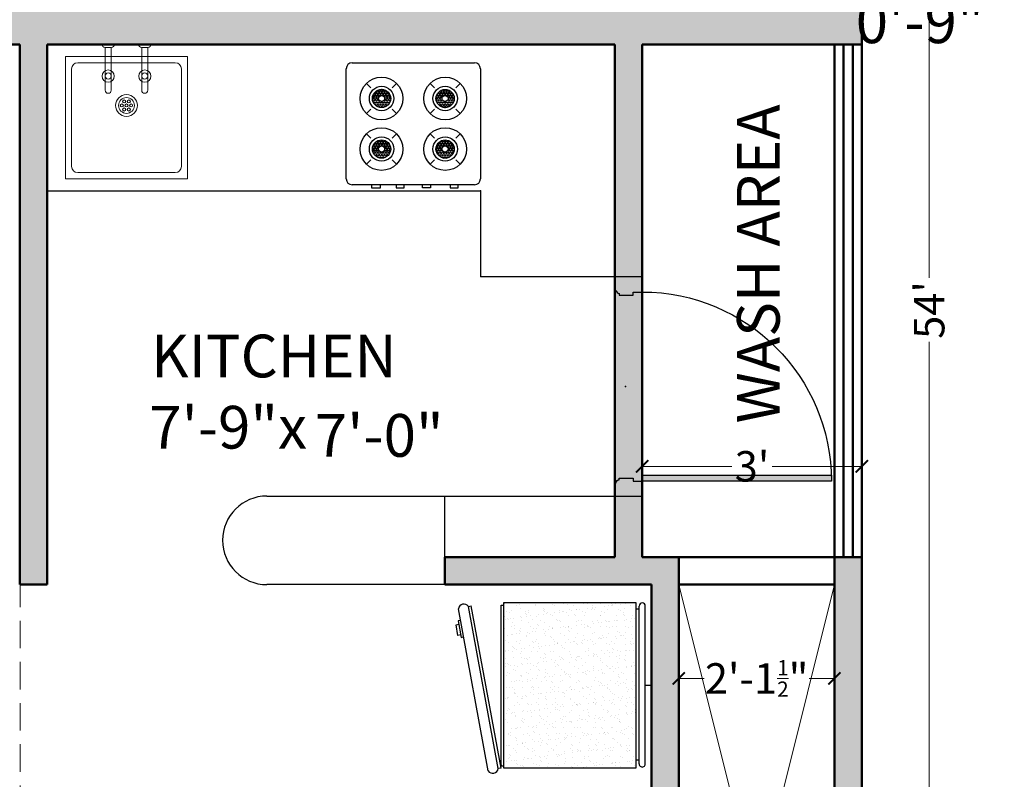
# Model space of a CAD drawing. Units: inches. Extents: x 4508 to 5907, y 877 to 1592.
# Tile 12 of 20: x 5392 to 5553, y 1174 to 1298. Entities that reach past the tile are written whole.
import ezdxf

# ---------------------------------------------------------------- set-up
doc = ezdxf.new("R2010")
doc.units = ezdxf.units.IN
doc.linetypes.add('DASHED', pattern=[0.75, 0.5, -0.25])
doc.layers.get('DEFPOINTS').update_dxf_attribs({"color": 8})
for name, color, linetype, lineweight in [('A-ANNO-DIMS', 2, 'Continuous', 18), ('A-ANNO-TEXT', 7, 'Continuous', 25), ('A-DOOR', 4, 'Continuous', 25), ('A-FLOR-CASE', 30, 'Continuous', 25), ('A-FLOR-FIXT', 8, 'Continuous', 18), ('A-FLOR-OVHD', 5, 'DASHED', 18), ('A-FLOR-SHFT', 8, 'Continuous', 18), ('A-WALL', 7, 'Continuous', 50), ('A-WALL-PATT', 8, 'Continuous', 13)]:
    doc.layers.add(name, color=color, linetype=linetype, lineweight=lineweight)
doc.layers.add('doors & windows', color=30, linetype='Continuous')
doc.layers.add('furniture', color=24, linetype='Continuous')
doc.styles.get("Standard").update_dxf_attribs({"font": 'arial.ttf'})
doc.dimstyles.new('details', dxfattribs={"dimtxt": 5, "dimasz": 2, "dimexe": 2, "dimexo": 3, "dimgap": 1, "dimtad": 0, "dimdec": 1, "dimzin": 0, "dimdsep": 46, "dimlunit": 4, "dimtxsty": 'Standard', "dimblk": 'ARCHTICK', "dimcen": 3, "dimclrd": 256, "dimclre": 256, "dimclrt": 256, "dimadec": 0, "dimazin": 0, "dimtfac": 0.5, "dimtdec": 1, "dimtofl": 0, "dimtmove": 0, "dimatfit": 3, "dimldrblk": 'CLOSEDBLANK', "dimfxl": 2, "dimtolj": 1, "dimtzin": 0, "dimlwd": -1, "dimlwe": -1, "dimarcsym": 0})
doc.dimstyles.new('text', dxfattribs={"dimtxt": 7, "dimasz": 0, "dimexe": 3, "dimexo": 3, "dimgap": 0, "dimtad": 1, "dimtih": 1, "dimtoh": 1, "dimzin": 3, "dimdsep": 46, "dimlunit": 4, "dimtxsty": 'Standard', "dimblk": 'CLOSEDBLANK', "dimcen": 3, "dimse1": 1, "dimse2": 1, "dimsd1": 1, "dimsd2": 1, "dimclrd": 256, "dimclre": 256, "dimclrt": 256, "dimadec": 0, "dimazin": 0, "dimtfac": 0.5, "dimtofl": 0, "dimtmove": 0, "dimatfit": 3, "dimfxl": 3, "dimtolj": 1, "dimtzin": 0, "dimlwd": -1, "dimlwe": -1, "dimarcsym": 0})

# ---------------------------------------------------------------- blocks, each defined once
blk = doc.blocks.new('_ArchTick')
at = {"color": 0, "linetype": 'ByBlock', "const_width": 0.15}
blk.add_lwpolyline([(-0.5, -0.5), (0.5, 0.5)], dxfattribs=at)
blk = doc.blocks.new('*D92')
at = {"layer": 'A-ANNO-DIMS', "color": 0, "transparency": 16777216}
for p, q in [((5499.9, 1202.7), (5499.9, 1188.32)), ((5525.4, 1202.7), (5525.4, 1188.32)), ((5499.9, 1190.32), (5504.05, 1190.32)), ((5525.4, 1190.32), (5521.25, 1190.32))]:
    blk.add_line(p, q, dxfattribs=at)
at = {"layer": 'DEFPOINTS', "color": 0, "transparency": 16777216}
for p in [(5499.9, 1205.7), (5525.4, 1205.7), (5499.9, 1190.32)]:
    blk.add_point(p, dxfattribs=at)
at = {"layer": 'A-ANNO-DIMS', "color": 0, "transparency": 16777216, "xscale": 2, "yscale": 2, "zscale": 2, "rotation": 180}
blk.add_blockref('_ArchTick', (5499.9, 1190.32), dxfattribs=at)
at = {"layer": 'A-ANNO-DIMS', "color": 0, "transparency": 16777216, "xscale": 2, "yscale": 2, "zscale": 2}
blk.add_blockref('_ArchTick', (5525.4, 1190.32), dxfattribs=at)
at = {"layer": 'A-ANNO-DIMS', "color": 0, "transparency": 16777216, "insert": (5512.65, 1190.32), "char_height": 5, "attachment_point": 5}
blk.add_mtext('\\A1;2\'-1{\\H0.5x;\\S1/2;}"', dxfattribs=at)
blk = doc.blocks.new('_ClosedBlank')
at = {"color": 0, "lineweight": -2}
for p, q in [((-1, 0.167), (0, 0)), ((-1, 0.167), (-1, -0.167)), ((0, 0), (-1, -0.167))]:
    blk.add_line(p, q, dxfattribs=at)
blk = doc.blocks.new('D1')
at = {"layer": 'doors & windows'}
h = blk.add_hatch(dxfattribs=at)
h.set_pattern_fill('DOTS', color=256, scale=2, angle=180, style=0)
h.set_pattern_definition([(180, (-2e-12, -4), (-0.0625, -0.125), [0, -0.125])])
h.paths.add_polyline_path([(2.5, 0), (3.5, 0), (3.5, 30.98, 0.008066), (2.5, 31)])
h = blk.add_hatch(dxfattribs=at)
h.set_pattern_fill('DOTS', color=256, scale=2, angle=180, style=0)
h.set_pattern_definition([(180, (0, -0.5), (-0.0625, -0.125), [0, -0.125])])
h.paths.add_polyline_path([(0, -4.5), (2.25, -4.5), (2.25, -4.25, 0.403966), (2.75, -3.75), (3, -3.75), (3, -1.5), (2.5, -1.5), (2.5, 0), (0, 0)])
h.paths.add_polyline_path([(36, -4.5), (36, 0), (33.5, 0), (33.5, -1.5), (33, -1.5), (33, -3.75), (33.25, -3.75, 0.403966), (33.75, -4.25), (33.75, -4.5)])
for p, q in [((0, 0), (0, -4.5)), ((36, 0), (36, -4.5))]:
    blk.add_line(p, q)
blk.add_lwpolyline([(3.5, 0), (3.5, 31), (2.5, 31), (2.5, 0)], close=True, dxfattribs=at)
for points in [[(3, -3.75), (3, -1.5), (2.5, -1.5), (2.5, 0), (0, 0)], [(33, -3.75), (33, -1.5), (33.5, -1.5), (33.5, 0), (36, 0)], [(0, -4.5), (2.25, -4.5)], [(36, -4.5), (33.75, -4.5)]]:
    blk.add_lwpolyline(points, dxfattribs=at)
for points in [[(2.25, -4.5), (2.25, -4.25, 0.403966), (2.75, -3.75), (3, -3.75)], [(33.75, -4.5), (33.75, -4.25, -0.403966), (33.25, -3.75), (33, -3.75)]]:
    blk.add_lwpolyline(points, format="xyb", dxfattribs=at)
at = {"layer": 'doors & windows', "ltscale": 6}
blk.add_arc((2.5, 0), 31, 0, 90, dxfattribs=at)
at = {"layer": 'doors & windows'}
blk.add_point((18, -2.75), dxfattribs=at)
blk = doc.blocks.new('*D93')
at = {"layer": 'A-ANNO-DIMS', "color": 0, "transparency": 16777216}
for p, q in [((5493.9, 1213.2), (5493.9, 1227.07)), ((5529.9, 1213.2), (5529.9, 1227.07)), ((5493.9, 1225.07), (5508.6, 1225.07)), ((5529.9, 1225.07), (5515.2, 1225.07))]:
    blk.add_line(p, q, dxfattribs=at)
at = {"layer": 'DEFPOINTS', "color": 0, "transparency": 16777216}
for p in [(5529.9, 1225.07), (5493.9, 1210.2), (5529.9, 1210.2)]:
    blk.add_point(p, dxfattribs=at)
at = {"layer": 'A-ANNO-DIMS', "color": 0, "transparency": 16777216, "xscale": 2, "yscale": 2, "zscale": 2, "rotation": 180}
blk.add_blockref('_ArchTick', (5493.9, 1225.07), dxfattribs=at)
at = {"layer": 'A-ANNO-DIMS', "color": 0, "transparency": 16777216, "xscale": 2, "yscale": 2, "zscale": 2}
blk.add_blockref('_ArchTick', (5529.9, 1225.07), dxfattribs=at)
at = {"layer": 'A-ANNO-DIMS', "color": 0, "transparency": 16777216, "insert": (5511.9, 1225.07), "char_height": 5, "attachment_point": 5}
blk.add_mtext("\\A1;3'", dxfattribs=at)
blk = doc.blocks.new('refrigerator')
at = {"layer": 'furniture'}
h = blk.add_hatch(dxfattribs=at)
h.set_pattern_fill('AR-SAND', color=256, angle=-90, style=0)
h.set_pattern_definition([(307.5, (-13.5104, -1), (1.926824, 0.06299), [0, -1.52, 0, -1.7, 0, -1.625]), (277.5, (-13.5104, -1), (2.82215, -1.76978), [0, -0.82, 0, -1.37, 0, -0.525]), (237.5, (-13.5104, 0.23), (0.00566, -3.11414), [0, -0.5, 0, -1.8, 0, -2.35]), (227.5, (-13.5104, 0.23), (0.87768, -3.00613), [0, -0.25, 0, -1.18, 0, -1.35])])
h.paths.add_polyline_path([(13.6, -24.16), (13.6, -2.56), (-13.51, -2.56), (-13.51, -24.16)])
for p, q in [((0, -1), (0, 0)), ((12.94, -1), (-12.94, -1)), ((-13.51, -2.56), (13.6, -2.56)), ((-13.51, -24.16), (-13.51, -2.56)), ((12.94, -2), (-12.94, -2)), ((-12.41, -2), (-12.41, -2.56)), ((12.29, -2), (12.29, -2.56)), ((13.6, -2.56), (13.6, -24.16)), ((13.6, -24.16), (-13.51, -24.16)), ((-13.07, -24.59), (-13.07, -24.16)), ((13.26, -24.59), (13.26, -24.16)), ((13.26, -24.59), (-13.07, -24.59)), ((13.6, -24.61), (-12.95, -29.5)), ((13.7, -25.1), (-12.85, -29.99)), ((13.07, -24.59), (13.26, -24.62)), ((13.26, -24.62), (13.07, -24.71)), ((13.6, -24.61), (13.7, -25.1)), ((14.06, -26.73), (-12.49, -31.62)), ((-12.85, -29.99), (-12.95, -29.5)), ((-10.58, -31.27), (-10.49, -31.65)), ((-10.49, -31.65), (-7.79, -31.16)), ((-9.87, -32.01), (-9.97, -31.56)), ((-8.13, -31.69), (-9.87, -32.01)), ((-8.23, -31.24), (-8.13, -31.69)), ((-7.79, -31.16), (-7.88, -30.77))]:
    blk.add_line(p, q, dxfattribs=at)
for centre, radius, start, end in [((-12.94, -1.5), 0.5, 90, 270), ((12.94, -1.5), 0.5, 270, 90), ((13.58, -25.98), 0.888, 302.2332, 82.2568), ((-12.38, -30.74), 0.888, 122.2332, 262.2568)]:
    blk.add_arc(centre, radius, start, end, dxfattribs=at)
blk = doc.blocks.new('*D95')
at = {"layer": 'DEFPOINTS', "color": 0, "transparency": 16777216}
for p in [(5445.95, 1205.7), (5452.67, 1205.7), (5443.65, 1103.7)]:
    blk.add_point(p, dxfattribs=at)
at = {"layer": 'A-ANNO-DIMS', "color": 0, "transparency": 16777216, "insert": (5452.67, 1138.42), "char_height": 7, "attachment_point": 5}
blk.add_mtext('\\A1;8\'-6"', dxfattribs=at)
blk = doc.blocks.new('sink')
for p, q in [((0, 0), (-24, 0)), ((0, 0), (0, 0)), ((-22, -3), (-2, -3)), ((-22, -23), (-22, -3)), ((-2, -3), (-2, -23)), ((-20, -4), (-4, -4)), ((-21, -21), (-21, -5)), ((-3, -5), (-3, -21)), ((-0.5, -9.5), (-7.5, -9.5)), ((-0.5, -9.5), (-0.5, -10.5)), ((0, -9), (0, -11)), ((-0.5, -10.5), (-7.5, -10.5)), ((-0.5, -15.5), (-7.5, -15.5)), ((-0.5, -15.5), (-0.5, -16.5)), ((0, -15), (0, -17)), ((-0.5, -16.5), (-7.5, -16.5)), ((-20, -22), (-4, -22)), ((-22, -23), (-2, -23))]:
    blk.add_line(p, q)
for centre, radius in [((-5.18, -10), 1), ((-5.18, -10), 0.5), ((-10, -13), 1.79), ((-10, -13), 1.29), ((-10.66, -12.62), 0.25), ((-10, -12.24), 0.25), ((-10, -13), 0.25), ((-9.34, -12.62), 0.25), ((-10.66, -13.38), 0.25), ((-10, -13.76), 0.25), ((-9.34, -13.38), 0.25), ((-5.18, -16), 1), ((-5.18, -16), 0.5)]:
    blk.add_circle(centre, radius)
for centre, radius, start, end in [((-20, -5), 1, 90, 180), ((-4, -5), 1, 0, 90), ((-7.5, -10), 0.5, 90, 270), ((0.01, -9.51), 0.511, 91.1728, 178.8272), ((0.01, -10.49), 0.511, 181.1728, 268.8272), ((-7.5, -16), 0.5, 90, 270), ((0.01, -15.51), 0.511, 91.1728, 178.8272), ((0.01, -16.49), 0.511, 181.1728, 268.8272), ((-20, -21), 1, 180, 270), ((-4, -21), 1, 270, 0)]:
    blk.add_arc(centre, radius, start, end)
blk = doc.blocks.new('stove')
at = {"layer": 'furniture'}
h = blk.add_hatch(dxfattribs=at)
h.set_pattern_fill('HEX', color=256, angle=180, style=0)
h.set_pattern_definition([(360, (22, 21.5), (1e-16, 0.2165064), [0.125, -0.25]), (120, (22, 21.5), (-0.1875, -0.1082532), [0.125, -0.25]), (60, (22.125, 21.5), (-0.1875, 0.1082532), [0.125, -0.25])])
h.paths.add_polyline_path([(5.36, 16.21, 1), (8.36, 16.21, 1)])
h.paths.add_polyline_path([(7.36, 16.21, -1), (6.36, 16.21, -1)], flags=16)
h = blk.add_hatch(dxfattribs=at)
h.set_pattern_fill('HEX', color=256, angle=180, style=0)
h.set_pattern_definition([(180, (2e-13, 21.5), (-1e-16, 0.2165064), [0.125, -0.25]), (60, (2e-13, 21.5), (0.1875, -0.1082532), [0.125, -0.25]), (120, (-0.125, 21.5), (0.1875, 0.1082532), [0.125, -0.25])])
h.paths.add_polyline_path([(13.64, 16.21, 1), (16.64, 16.21, 1)])
h.paths.add_polyline_path([(15.64, 16.21, -1), (14.64, 16.21, -1)], flags=16)
h = blk.add_hatch(dxfattribs=at)
h.set_pattern_fill('HEX', color=256, angle=180, style=0)
h.set_pattern_definition([(360, (22, 0.5), (-1e-16, -0.2165064), [0.125, -0.25]), (240, (22, 0.5), (-0.1875, 0.1082532), [0.125, -0.25]), (300, (22.125, 0.5), (-0.1875, -0.1082532), [0.125, -0.25])])
h.paths.add_polyline_path([(8.36, 5.79, 1), (5.36, 5.79, 1)])
h.paths.add_polyline_path([(6.36, 5.79, -1), (7.36, 5.79, -1)], flags=16)
h = blk.add_hatch(dxfattribs=at)
h.set_pattern_fill('HEX', color=256, angle=180, style=0)
h.set_pattern_definition([(180, (2e-13, 0.5), (1e-16, -0.2165064), [0.125, -0.25]), (300, (2e-13, 0.5), (0.1875, 0.1082532), [0.125, -0.25]), (240, (-0.125, 0.5), (0.1875, -0.1082532), [0.125, -0.25])])
h.paths.add_polyline_path([(16.64, 5.79, 1), (13.64, 5.79, 1)])
h.paths.add_polyline_path([(14.64, 5.79, -1), (15.64, 5.79, -1)], flags=16)
for p, q in [((1, 1), (1, 21)), ((2, 22), (20, 22)), ((21, 21), (21, 1)), ((1, 17.86), (0.5, 17.86)), ((0.5, 17.86), (0.5, 16.36)), ((4.39, 18.69), (5.1, 17.98)), ((8.63, 17.98), (9.34, 18.69)), ((13.37, 17.98), (12.66, 18.69)), ((17.61, 18.69), (16.9, 17.98)), ((0.5, 16.36), (1, 16.36)), ((0.5, 13.8), (0.5, 12.5)), ((1, 13.8), (0.5, 13.8)), ((4.39, 13.74), (5.1, 14.45)), ((8.63, 14.45), (9.34, 13.74)), ((13.37, 14.45), (12.66, 13.74)), ((17.61, 13.74), (16.9, 14.45)), ((0.5, 12.5), (1, 12.5)), ((0.5, 9.5), (1, 9.5)), ((0.5, 8.2), (0.5, 9.5)), ((1, 8.2), (0.5, 8.2)), ((4.39, 8.26), (5.1, 7.55)), ((8.63, 7.55), (9.34, 8.26)), ((13.37, 7.55), (12.66, 8.26)), ((17.61, 8.26), (16.9, 7.55)), ((0.5, 4.94), (0.5, 3.64)), ((1, 4.94), (0.5, 4.94)), ((0.5, 3.64), (1, 3.64)), ((4.39, 3.31), (5.1, 4.02)), ((8.63, 4.02), (9.34, 3.31)), ((13.37, 4.02), (12.66, 3.31)), ((17.61, 3.31), (16.9, 4.02)), ((20, 0), (2, 0))]:
    blk.add_line(p, q, dxfattribs=at)
for centre, radius in [((6.86, 16.21), 3.5), ((15.14, 16.21), 3.5), ((6.86, 16.21), 2), ((15.14, 16.21), 2), ((6.86, 16.21), 1.5), ((6.86, 16.21), 0.5), ((15.14, 16.21), 1.5), ((15.14, 16.21), 0.5), ((6.86, 5.79), 3.5), ((15.14, 5.79), 3.5), ((6.86, 5.79), 2), ((6.86, 5.79), 1.5), ((15.14, 5.79), 2), ((15.14, 5.79), 1.5), ((6.86, 5.79), 0.5), ((15.14, 5.79), 0.5)]:
    blk.add_circle(centre, radius, dxfattribs=at)
for centre, start, end in [((2, 21), 90, 180), ((20, 21), 0, 90), ((2, 1), 180, 270), ((20, 1), 270, 0)]:
    blk.add_arc(centre, 1, start, end, dxfattribs=at)
at = {"layer": 'furniture', "ltscale": 9}
blk.add_point((0, 0), dxfattribs=at)
blk = doc.blocks.new('*D96')
at = {"layer": 'DEFPOINTS', "color": 0, "transparency": 16777216}
for p in [(5396.4, 1237.32), (5396.4, 1235.92), (5489.4, 1236.4)]:
    blk.add_point(p, dxfattribs=at)
at = {"layer": 'A-ANNO-DIMS', "color": 0, "transparency": 16777216, "insert": (5426.06, 1237.32), "char_height": 7, "attachment_point": 5}
blk.add_mtext('\\A1;       KITCHEN\\P7\'-9"x', dxfattribs=at)
blk = doc.blocks.new('*D97')
at = {"layer": 'DEFPOINTS', "color": 0, "transparency": 16777216}
for p in [(5444.83, 1294.2), (5450.81, 1294.2), (5442.54, 1210.2)]:
    blk.add_point(p, dxfattribs=at)
at = {"layer": 'A-ANNO-DIMS', "color": 0, "transparency": 16777216, "insert": (5450.81, 1230.15), "char_height": 7, "attachment_point": 5}
blk.add_mtext('\\A1;7\'-0"', dxfattribs=at)
blk = doc.blocks.new('*D98')
at = {"layer": 'DEFPOINTS', "color": 0, "transparency": 16777216}
for p in [(5255.4, 1205.15), (5391.9, 1205.7), (5255.4, 1203.74)]:
    blk.add_point(p, dxfattribs=at)
at = {"layer": 'A-ANNO-DIMS', "color": 0, "transparency": 16777216, "insert": (5316.09, 1205.15), "char_height": 7, "attachment_point": 5}
blk.add_mtext('\\A1;          HALL\\P11\'-4{\\H0.5x;\\S1/2;}"x', dxfattribs=at)
blk = doc.blocks.new('*D113')
at = {"layer": 'A-ANNO-DIMS', "color": 0, "transparency": 16777216}
for p, q in [((5532.9, 1574.7), (5542.92, 1574.7)), ((5540.92, 1574.7), (5540.92, 1255.95)), ((5540.92, 926.7), (5540.92, 1245.46)), ((5532.9, 926.7), (5542.92, 926.7))]:
    blk.add_line(p, q, dxfattribs=at)
at = {"layer": 'DEFPOINTS', "color": 0, "transparency": 16777216}
for p in [(5529.9, 1574.7), (5540.92, 1574.7), (5529.9, 926.7)]:
    blk.add_point(p, dxfattribs=at)
at = {"layer": 'A-ANNO-DIMS', "color": 0, "transparency": 16777216, "xscale": 2, "yscale": 2, "zscale": 2}
for p, rotation in [((5540.92, 1574.7), 90), ((5540.92, 926.7), 270)]:
    blk.add_blockref('_ArchTick', p, dxfattribs=dict(at, rotation=rotation))
at = {"layer": 'A-ANNO-DIMS', "color": 0, "transparency": 16777216, "insert": (5540.92, 1250.7), "char_height": 5, "attachment_point": 5, "rotation": 90}
blk.add_mtext("\\A1;54'", dxfattribs=at)
blk = doc.blocks.new('*D191')
at = {"layer": 'DEFPOINTS', "color": 0, "transparency": 16777216}
for p in [(5539.438529, 1302.416611), (5579.745522, 1302.416611), (5579.787188, 1293.416611)]:
    blk.add_point(p, dxfattribs=at)
at = {"layer": 'A-ANNO-DIMS', "transparency": 16777216, "insert": (5539.438529, 1297.916611), "char_height": 7, "attachment_point": 5}
blk.add_mtext('\\A1;0\'-9"', dxfattribs=at)

msp = doc.modelspace()

# ---------------------------------------------------------------- hatches: boundary and pattern name
at = {"layer": 'A-WALL-PATT'}
h = msp.add_hatch(color=256, dxfattribs=at)
h.dxf.hatch_style = 1
h.paths.add_polyline_path([(5529.903, 1303.204), (5388.02, 1303.204), (5388.02, 1294.204), (5391.903, 1294.204), (5391.903, 1205.704), (5396.403, 1205.704), (5396.403, 1294.204), (5489.403, 1294.204), (5489.403, 1256.139), (5493.903, 1256.139), (5493.903, 1294.204), (5529.903, 1294.204)], flags=17)
h.paths.add_polyline_path([(5346.02, 1303.204), (5322.903, 1303.204), (5322.903, 1321.388), (5313.903, 1321.388), (5313.903, 1303.204), (5259.903, 1303.204), (5259.903, 1381.204), (5313.903, 1381.204), (5313.903, 1359.674), (5322.903, 1359.674), (5322.903, 1381.204), (5338.979, 1381.204), (5338.979, 1390.204), (5331.903, 1390.204), (5331.903, 1442.704), (5255.403, 1442.704), (5255.403, 1570.204), (5387.403, 1570.204), (5387.403, 1541.271), (5391.903, 1541.271), (5391.903, 1570.204), (5483.403, 1570.204), (5483.403, 1498.204), (5391.903, 1498.204), (5391.903, 1509.559), (5387.403, 1509.559), (5387.403, 1390.204), (5380.979, 1390.204), (5380.979, 1381.204), (5387.403, 1381.204), (5529.903, 1381.204), (5529.903, 1498.204), (5487.903, 1498.204), (5487.903, 1570.204), (5529.903, 1570.204), (5529.903, 1574.704), (5250.903, 1574.704), (5250.903, 991.204), (5310.903, 991.204), (5310.903, 926.704), (5529.903, 926.704), (5529.903, 1210.204), (5525.403, 1210.204), (5525.403, 1103.704), (5499.903, 1103.704), (5499.903, 1210.204), (5493.903, 1210.204), (5493.903, 1256.139), (5489.403, 1256.139), (5489.403, 1210.204), (5461.584, 1210.204), (5461.584, 1205.704), (5495.403, 1205.704), (5495.403, 1103.704), (5436.903, 1103.704), (5436.903, 1051.204), (5391.954, 1051.204), (5391.954, 1103.03), (5391.954, 1107.53), (5255.403, 1108.204), (5255.403, 1294.204), (5346.02, 1294.204)])
h.paths.add_polyline_path([(5255.403, 1390.204), (5255.403, 1398.204), (5255.403, 1438.204), (5257.903, 1438.204), (5258.903, 1438.204), (5327.403, 1438.204), (5327.403, 1390.204), (5325.903, 1390.204)], flags=16)
h.paths.add_polyline_path([(5288.757, 1390.704), (5288.757, 1390.204), (5292.173, 1390.204), (5292.173, 1390.704)], flags=0)
h.paths.add_polyline_path([(5289.965, 1391.606), (5289.965, 1396.645), (5289.903, 1396.645), (5289.903, 1397.319), (5288.849, 1398.862), (5288.849, 1398.8), (5288.983, 1398.748), (5288.983, 1399.204), (5289.091, 1399.204), (5292.081, 1399.204), (5292.081, 1398.665), (5291.946, 1398.665), (5291.027, 1397.319), (5291.027, 1396.645), (5290.965, 1396.645), (5290.965, 1391.606)], flags=0)
h.paths.add_polyline_path([(5288.849, 1399.069, 2.6374395), (5289.056, 1398.835), (5289.117, 1399.087, 0.9346155)], flags=0)
h.paths.add_polyline_path([(5290.061, 1398.665), (5290.061, 1399.204), (5290.038, 1398.975)], flags=0)
h.paths.add_polyline_path([(5291.946, 1398.934, -1), (5291.946, 1398.665)], flags=0)
h.paths.add_polyline_path([(5289.414, 1398.967), (5289.414, 1399.204), (5289.63, 1399.204), (5289.63, 1398.363), (5290.051, 1397.184), (5290.76, 1397.184), (5290.869, 1398.665), (5290.869, 1399.204), (5290.815, 1398.665), (5290.815, 1399.204), (5291.462, 1399.204), (5291.462, 1398.816), (5290.879, 1397.184), (5290.051, 1397.184)], flags=0)
h.paths.add_polyline_path([(5273.903, 1392.056), (5269.591, 1392.056, 0.0901028), (5265.544, 1392.842), (5265.511, 1392.034, -0.3516542), (5265.903, 1391.546, -1), (5264.903, 1391.546, -0.3042165), (5265.213, 1392.008), (5265.167, 1392.84, 0.0880132), (5261.215, 1392.056), (5256.903, 1392.056), (5256.903, 1398.704, -0.4142136), (5259.403, 1401.204), (5271.403, 1401.204, -0.4142136), (5273.903, 1398.704)], flags=0)
h.paths.add_polyline_path([(5263.726, 1395.073, -1), (5267.08, 1395.073, -1)], flags=0)
h.paths.add_polyline_path([(5264.434, 1395.073, -0.695521), (5265.153, 1395.073, -1.1408699), (5265.403, 1395.585, -0.7522125), (5265.403, 1396.25, 0.3674806)], flags=0)
h.paths.add_polyline_path([(5265.153, 1394.399, -1), (5265.653, 1394.399, -1)], flags=0)
h.paths.add_polyline_path([(5265.905, 1395.077, -1), (5266.405, 1395.077, -1)], flags=0)
h.paths.add_polyline_path([(5307.994, 1403.113, -1), (5307.994, 1417.295), (5318.794, 1417.295, -0.4142136), (5319.794, 1416.295), (5320.794, 1416.295, -0.4142136), (5321.794, 1417.295), (5324.903, 1417.295, -0.4142136), (5325.903, 1416.295), (5325.903, 1404.113, -0.4142136), (5324.903, 1403.113), (5321.794, 1403.113, -0.4142136), (5320.794, 1404.113), (5319.794, 1404.113, -0.4142136), (5318.794, 1403.113)], flags=0)
h.paths.add_polyline_path([(5307.836, 1405.113, -1), (5307.836, 1415.295), (5315.591, 1415.295, -0.4142136), (5317.532, 1413.353), (5317.532, 1407.054, -0.4142136), (5315.591, 1405.113)], flags=0)
h.paths.add_polyline_path([(5312.032, 1408.204, -1), (5312.032, 1412.204), (5315.032, 1412.204, -0.4142136), (5316.032, 1411.204), (5316.032, 1409.204, -0.4142136), (5315.032, 1408.204)], flags=0)
h.paths.add_polyline_path([(5391.903, 1385.704), (5391.903, 1493.704), (5525.403, 1493.704), (5525.403, 1385.704)], flags=16)
h.paths.add_polyline_path([(5422.641, 1390.704), (5422.641, 1465.704, -0.9426302), (5422.641, 1467.704), (5494.547, 1467.704, -1), (5494.665, 1465.704), (5494.665, 1390.704, -0.9426302), (5494.665, 1388.704), (5422.759, 1388.704, -1)], flags=0)
h.paths.add_polyline_path([(5427.52, 1395.749, -0.0238564), (5427.614, 1403.949, 0.0884332), (5427.476, 1405.056, 0.0506693), (5427.273, 1405.463, -0.8716827), (5427.713, 1405.835, 0.0268855), (5431.815, 1405.361, 0.0306964), (5436.289, 1405.361, -0.0263641), (5445.798, 1405.259, 0.075811), (5450.408, 1405.53, 0.0687062), (5454.457, 1405.903, -1.0086747), (5454.781, 1405.482, 0.0692081), (5454.389, 1400.959, -0.0519468), (5454.356, 1394.996, 0.1195012), (5454.627, 1392.895, 0.0143508), (5454.796, 1392.489, -0.6962059), (5454.42, 1392.118, 0.1574808), (5448.747, 1392.794, -0.025536), (5432.749, 1392.774, 0.0920085), (5427.781, 1392.048, -0.9384848), (5427.137, 1392.455, 0.0063894), (5427.314, 1392.79, 0.0472995)], flags=0)
h.paths.add_polyline_path([(5426.125, 1411.372, 0.0617649), (5428.641, 1412.201), (5428.641, 1465.704), (5488.665, 1465.704), (5488.665, 1412.363, 0.2363822), (5467.6, 1412.052, -0.2252042)], flags=0)
h.paths.add_polyline_path([(5391.903, 1490.204), (5391.903, 1491.204), (5422.903, 1491.204), (5422.903, 1490.204)], flags=0)
h.paths.add_polyline_path([(5462.545, 1392.771, 0.1270318), (5462.866, 1394.996, -0.0519468), (5462.832, 1400.959, 0.0692081), (5462.441, 1405.482, -1.0086747), (5462.765, 1405.903, 0.0857004), (5471.424, 1405.259, -0.0263641), (5480.932, 1405.361, 0.0306964), (5485.407, 1405.361, 0.0268855), (5489.509, 1405.835, -0.8716827), (5489.949, 1405.463, 0.0506693), (5489.746, 1405.056, 0.0884332), (5489.608, 1403.949, -0.0238564), (5489.702, 1395.749, 0.0472995), (5489.908, 1392.79, 0.0063894), (5490.085, 1392.455, -0.9384848), (5489.441, 1392.048, 0.0920085), (5484.473, 1392.774, -0.025536), (5468.475, 1392.794, 0.1574808), (5462.802, 1392.118, -0.6962059), (5462.426, 1392.489, 0.0100173), (5462.546, 1392.771)], flags=0)
h.paths.add_polyline_path([(5387.454, 1103.03), (5387.454, 1100.53), (5387.454, 1099.53), (5387.454, 995.03), (5387.454, 991.204), (5391.954, 991.204), (5391.954, 1046.704), (5525.403, 1046.704), (5525.403, 931.182), (5391.954, 930.53), (5391.954, 960.53), (5387.454, 960.53), (5387.454, 930.53), (5315.403, 930.53), (5315.403, 991.204), (5323.403, 991.204), (5387.454, 991.204), (5387.454, 995.03), (5255.403, 995.704), (5255.403, 1103.704)], flags=16)
h.paths.add_polyline_path([(5379.264, 1062.889), (5379.264, 1060.156), (5385.764, 1061.889, -0.4526903), (5385.764, 1059.889), (5379.264, 1059.889), (5379.264, 1055.156), (5385.764, 1056.889, -0.4526903), (5385.764, 1054.889), (5379.264, 1054.889), (5379.264, 1050.156), (5385.764, 1051.889, -0.4526903), (5385.764, 1049.889), (5379.264, 1049.889), (5379.264, 1010.156), (5385.764, 1011.889, -0.4526903), (5385.764, 1009.889), (5379.264, 1009.889), (5379.264, 1005.156), (5385.764, 1006.889, -0.4526903), (5385.764, 1004.889), (5379.264, 1004.889), (5379.264, 1000.156), (5385.764, 1001.889, -0.4526903), (5385.764, 999.889), (5378.264, 999.889), (5370.764, 997.889, -0.6674863), (5370.764, 999.889), (5377.264, 999.889), (5377.264, 1004.623), (5370.764, 1002.889, -0.6674863), (5370.764, 1004.889), (5377.264, 1004.889), (5377.264, 1009.623), (5370.764, 1007.889, -0.6674863), (5370.764, 1009.889), (5377.264, 1009.889), (5377.264, 1049.623), (5370.764, 1047.889, -0.6674863), (5370.764, 1049.889), (5377.264, 1049.889), (5377.264, 1054.623), (5370.764, 1052.889, -0.6674863), (5370.764, 1054.889), (5377.264, 1054.889), (5377.264, 1059.623), (5370.764, 1057.889, -0.6674863), (5370.764, 1059.889), (5377.264, 1059.889), (5377.264, 1062.889)], flags=0)
h.paths.add_polyline_path([(5287.641, 1000.704), (5359.665, 1000.704), (5359.665, 1018.212, 0.3202856), (5332.6, 1022.052, -0.246494), (5287.641, 1023.128)], flags=0)
h.paths.add_polyline_path([(5359.547, 1077.704, -1), (5359.665, 1075.704), (5353.665, 1075.704), (5353.665, 1063.704), (5293.641, 1063.704), (5293.641, 1075.704), (5287.759, 1075.704, -1), (5287.641, 1077.704)], flags=0)
h.paths.add_polyline_path([(5441.403, 1099.204), (5525.403, 1099.204), (5525.403, 1051.204), (5441.403, 1051.204), (5441.403, 1059.204)], flags=16)
h.paths.add_polyline_path([(5441.403, 1096.704), (5466.403, 1096.704), (5466.403, 1095.704), (5441.403, 1095.704)], flags=0)
h.paths.add_polyline_path([(5445.403, 1062.204), (5457.403, 1062.204, -0.4142136), (5459.903, 1059.704), (5459.903, 1053.056), (5455.591, 1053.056, 0.0901028), (5451.544, 1053.842), (5451.511, 1053.034, -0.3516542), (5451.903, 1052.546, -1), (5450.903, 1052.546, -0.3042165), (5451.213, 1053.008), (5451.167, 1053.84, 0.0880132), (5447.215, 1053.056), (5442.903, 1053.056), (5442.903, 1059.704, -0.4142136)], flags=0)
h.paths.add_polyline_path([(5453.08, 1056.073, -1), (5449.726, 1056.073, -1)], flags=0)
h.paths.add_polyline_path([(5292.713, 1015.835, 0.0268855), (5296.815, 1015.361, 0.0306964), (5301.289, 1015.361, -0.0263641), (5310.798, 1015.259, 0.075811), (5315.408, 1015.53, 0.0687062), (5319.457, 1015.903, -1.0086747), (5319.781, 1015.482, 0.0692081), (5319.389, 1010.959, -0.0519468), (5319.356, 1004.996, 0.1195012), (5319.627, 1002.895, 0.0143508), (5319.796, 1002.489, -0.6962059), (5319.42, 1002.118, 0.1574808), (5313.747, 1002.794, -0.025536), (5297.749, 1002.774, 0.0920085), (5292.781, 1002.048, -0.9384848), (5292.137, 1002.455, 0.0063894), (5292.314, 1002.79, 0.0472995), (5292.52, 1005.749, -0.0238564), (5292.614, 1013.949, 0.0884332), (5292.476, 1015.056, 0.0506693), (5292.273, 1015.463, -0.8716827)], flags=0)
h.paths.add_polyline_path([(5450.434, 1056.073, -0.695521), (5451.153, 1056.073, -1.1408699), (5451.403, 1056.585, -0.7522125), (5451.403, 1057.25, 0.3674806)], flags=0)
h.paths.add_polyline_path([(5327.765, 1015.903, 0.0857004), (5336.424, 1015.259, -0.0263641), (5345.932, 1015.361, 0.0306964), (5350.407, 1015.361, 0.0268855), (5354.509, 1015.835, -0.8716827), (5354.949, 1015.463, 0.0506693), (5354.746, 1015.056, 0.0884332), (5354.608, 1013.949, -0.0238564), (5354.702, 1005.749, 0.0472995), (5354.908, 1002.79, 0.0063894), (5355.085, 1002.455, -0.9384848), (5354.441, 1002.048, 0.0920085), (5349.473, 1002.774, -0.025536), (5333.475, 1002.794, 0.1574808), (5327.802, 1002.118, -0.6962059), (5327.426, 1002.489, 0.0100173), (5327.546, 1002.771), (5327.545, 1002.771, 0.1270318), (5327.866, 1004.996, -0.0519468), (5327.832, 1010.959, 0.0692081), (5327.441, 1015.482, -1.0086747)], flags=0)
h.paths.add_polyline_path([(5452.405, 1056.077, -1), (5451.905, 1056.077, -1)], flags=0)
h.paths.add_polyline_path([(5451.653, 1055.399, -1), (5451.153, 1055.399, -1)], flags=0)
h.paths.add_polyline_path([(5472.958, 1051.704), (5472.958, 1051.204), (5476.374, 1051.204), (5476.374, 1051.704)], flags=0)
h.paths.add_polyline_path([(5476.282, 1060.204), (5476.282, 1059.665), (5476.147, 1059.665), (5475.228, 1058.319), (5475.228, 1057.645), (5475.166, 1052.606), (5474.166, 1052.606), (5474.166, 1057.645), (5474.104, 1057.645), (5474.104, 1058.319), (5473.05, 1059.862), (5473.05, 1059.8), (5473.184, 1059.748), (5473.184, 1060.204), (5473.292, 1060.204)], flags=0)
h.paths.add_polyline_path([(5473.05, 1060.069, 2.6374395), (5473.257, 1059.835), (5473.318, 1060.087, 0.9346155)], flags=0)
h.paths.add_polyline_path([(5473.831, 1060.204), (5473.831, 1059.363), (5474.252, 1058.184), (5474.371, 1058.184), (5474.262, 1059.665), (5474.262, 1060.204)], flags=0)
h.paths.add_polyline_path([(5475.501, 1060.204), (5475.501, 1059.363), (5475.555, 1059.514), (5475.555, 1060.204)], flags=0)
h.paths.add_polyline_path([(5474.855, 1060.204), (5474.908, 1060.127), (5474.908, 1060.204), (5474.855, 1059.665)], flags=0)
h.paths.add_polyline_path([(5476.147, 1059.934, -1), (5476.147, 1059.665)], flags=0)
h.paths.add_polyline_path([(5474.693, 1060.204), (5475.178, 1059.511), (5475.178, 1060.204), (5475.285, 1059.934), (5475.285, 1060.204), (5475.178, 1059.665), (5475.178, 1060.204), (5475.07, 1059.665), (5475.07, 1060.204), (5474.962, 1059.665), (5474.962, 1060.204), (5474.693, 1059.306)], flags=0)
h.paths.add_polyline_path([(5474.747, 1060.204), (5474.37, 1059.45), (5474.37, 1060.204), (5474.424, 1060.096), (5474.424, 1060.204), (5474.747, 1059.665)], flags=0)
h.paths.add_polyline_path([(5476.04, 1059.665), (5476.04, 1060.204), (5476.094, 1059.665), (5476.094, 1060.204)], flags=0)
h.paths.add_polyline_path([(5505.994, 1082.295), (5516.794, 1082.295, -0.4142136), (5517.794, 1081.295), (5518.794, 1081.295, -0.4142136), (5519.794, 1082.295), (5522.903, 1082.295, -0.4142136), (5523.903, 1081.295), (5523.903, 1069.113, -0.4142136), (5522.903, 1068.113), (5519.794, 1068.113, -0.4142136), (5518.794, 1069.113), (5517.794, 1069.113, -0.4142136), (5516.794, 1068.113), (5505.994, 1068.113, -1)], flags=0)
h.paths.add_polyline_path([(5505.836, 1080.295), (5513.591, 1080.295, -0.4142136), (5515.532, 1078.353), (5515.532, 1072.054, -0.4142136), (5513.591, 1070.113), (5505.836, 1070.113, -1)], flags=0)
h.paths.add_polyline_path([(5520.403, 963.695), (5520.403, 1035.72), (5502.895, 1035.72, 0.3202856), (5499.055, 1008.654, -0.246494), (5497.978, 963.695)], flags=0)
h.paths.add_polyline_path([(5445.403, 1035.72), (5445.403, 1029.72), (5457.403, 1029.72), (5457.403, 969.695), (5445.403, 969.695), (5445.403, 963.814, -1), (5443.403, 963.695), (5443.403, 1035.602, -1)], flags=0)
h.paths.add_polyline_path([(5510.032, 1077.204), (5513.032, 1077.204, -0.4142136), (5514.032, 1076.204), (5514.032, 1074.204, -0.4142136), (5513.032, 1073.204), (5510.032, 1073.204, -1)], flags=0)
h.paths.add_polyline_path([(5317.255, 989.704), (5323.903, 989.704, -0.4142136), (5326.403, 987.204), (5326.403, 975.204, -0.4142136), (5323.903, 972.704), (5317.255, 972.704), (5317.255, 977.016, 0.0901028), (5318.041, 981.063), (5317.233, 981.096, -0.8964437), (5316.245, 981.204, -0.8220123), (5317.207, 981.394), (5318.04, 981.44, 0.0880132), (5317.255, 985.392)], flags=0)
h.paths.add_polyline_path([(5321.949, 981.204, -1), (5318.594, 981.204, -1)], flags=0)
h.paths.add_polyline_path([(5362.454, 988.03), (5387.454, 988.03), (5387.454, 990.53), (5391.954, 990.53), (5391.704, 988.289, -0.4090807), (5391.204, 987.78), (5391.204, 987.53), (5388.954, 987.53), (5388.954, 988.03), (5387.454, 988.03), (5387.454, 987.03), (5362.474, 987.03, 0.4025427), (5387.454, 963.03), (5388.954, 963.03), (5388.954, 963.53), (5391.195, 963.28, -0.4142136), (5391.704, 962.771), (5391.954, 960.53), (5391.954, 962.78), (5391.704, 962.78, 0.4090807), (5391.195, 963.28), (5388.954, 963.53), (5388.954, 963.03), (5387.454, 963.03, -0.4025427), (5362.474, 987.03), (5362.454, 987.03)], flags=0)
h.paths.add_polyline_path([(5321.285, 981.204, -0.6555366), (5320.522, 981.204, -1.1195284), (5320.275, 980.701, -1.3500746), (5320.279, 980.026, 0.3749463)], flags=0)
h.paths.add_polyline_path([(5320.022, 981.923, -1), (5320.522, 981.923, -1)], flags=0)
h.paths.add_polyline_path([(5319.348, 981.204, -1), (5319.848, 981.204, -1)], flags=0)
h.paths.add_polyline_path([(5507.157, 1030.662, -0.0238564), (5515.358, 1030.756, 0.0472995), (5518.317, 1030.962, 0.0063894), (5518.652, 1031.139, -0.9384848), (5519.059, 1030.495, 0.0920085), (5518.333, 1025.527, -0.025536), (5518.313, 1009.53, 0.1574808), (5518.989, 1003.857, -0.6962059), (5518.618, 1003.48, 0.0100173), (5518.335, 1003.601), (5518.335, 1003.6, 0.1270318), (5516.111, 1003.921, -0.0519468), (5510.148, 1003.887, 0.0692081), (5505.624, 1003.495, -1.0086747), (5505.204, 1003.819, 0.0857004), (5505.848, 1012.479, -0.0263641), (5505.746, 1021.987, 0.0306964), (5505.746, 1026.462, 0.0268855), (5505.272, 1030.563, -0.8716827), (5505.644, 1031.004, 0.0506693), (5506.051, 1030.801, 0.0884332)], flags=0)
h.paths.add_polyline_path([(5368.045, 945.621), (5378.845, 945.621, -0.4142136), (5379.845, 944.621), (5380.845, 944.621, -0.4142136), (5381.845, 945.621), (5384.954, 945.621, -0.4142136), (5385.954, 944.621), (5385.954, 932.439, -0.4142136), (5384.954, 931.439), (5381.845, 931.439, -0.4142136), (5380.845, 932.439), (5379.845, 932.439, -0.4142136), (5378.845, 931.439), (5368.045, 931.439, -1)], flags=0)
h.paths.add_polyline_path([(5327.31, 931.03), (5327.31, 930.53), (5330.726, 930.53), (5330.726, 931.03)], flags=0)
h.paths.add_polyline_path([(5330.634, 939.53), (5330.634, 938.991), (5330.499, 938.991), (5329.579, 937.645), (5329.579, 936.971), (5329.518, 936.971), (5329.518, 931.933), (5328.518, 931.933), (5328.518, 936.971), (5328.456, 936.971), (5328.456, 937.645), (5327.402, 939.189), (5327.402, 939.126), (5327.536, 939.074), (5327.536, 939.53), (5327.644, 939.53)], flags=0)
h.paths.add_polyline_path([(5327.402, 939.395, 2.6374395), (5327.609, 939.161), (5327.67, 939.414, 0.9346155)], flags=0)
h.paths.add_polyline_path([(5328.021, 939.142), (5328.021, 939.53), (5327.967, 939.53), (5327.967, 939.293)], flags=0)
h.paths.add_polyline_path([(5328.614, 939.53), (5328.614, 938.991), (5328.723, 937.51), (5329.313, 937.51), (5329.422, 938.991), (5329.422, 939.53), (5329.368, 938.991), (5329.368, 939.53)], flags=0)
h.paths.add_polyline_path([(5329.853, 939.53), (5329.853, 938.689), (5329.907, 938.84), (5329.907, 939.53)], flags=0)
h.paths.add_polyline_path([(5330.499, 939.261, -1), (5330.499, 938.991)], flags=0)
h.paths.add_polyline_path([(5367.887, 943.621), (5375.641, 943.621, -0.4142136), (5377.583, 941.68), (5377.583, 935.38, -0.4142136), (5375.641, 933.439), (5367.887, 933.439, -1)], flags=0)
h.paths.add_polyline_path([(5509.267, 947.14), (5509.267, 939.64), (5511.267, 932.14, -0.4526903), (5509.267, 932.14), (5509.267, 938.64), (5504.534, 938.64), (5506.267, 932.14, -0.4526903), (5504.267, 932.14), (5504.267, 938.64), (5499.534, 938.64), (5501.267, 932.14, -0.4526903), (5499.267, 932.14), (5499.267, 938.64), (5459.534, 938.64), (5461.267, 932.14, -0.4526903), (5459.267, 932.14), (5459.267, 938.64), (5454.534, 938.64), (5456.267, 932.14, -0.4526903), (5454.267, 932.14), (5454.267, 938.64), (5449.534, 938.64), (5451.267, 932.14, -0.4526903), (5449.267, 932.14), (5449.267, 939.64), (5447.267, 947.14, -0.3030853), (5448.267, 947.808), (5508.266, 947.808, -0.3032033)], flags=0)
h.paths.add_polyline_path([(5510.148, 995.444, -0.0519468), (5516.111, 995.41, 0.1195012), (5518.212, 995.681, 0.0143508), (5518.618, 995.851, -0.6962059), (5518.989, 995.474, 0.1574808), (5518.313, 989.801, -0.025536), (5518.333, 973.804, 0.0920085), (5519.059, 968.836, -0.9384848), (5518.652, 968.192, 0.0063894), (5518.317, 968.369, 0.0472995), (5515.358, 968.575, -0.0238564), (5507.157, 968.669, 0.0884332), (5506.051, 968.531, 0.0506693), (5505.644, 968.327, -0.8716827), (5505.272, 968.768, 0.0268855), (5505.746, 972.869, 0.0306964), (5505.746, 977.344, -0.0263641), (5505.848, 986.852, 0.075811), (5505.576, 991.462, 0.0687062), (5505.204, 995.512, -1.0086747), (5505.624, 995.836, 0.0692081)], flags=0)
h.paths.add_polyline_path([(5372.083, 940.53), (5375.083, 940.53, -0.4142136), (5376.083, 939.53), (5376.083, 937.53, -0.4142136), (5375.083, 936.53), (5372.083, 936.53, -1)], flags=0)
h.paths.add_polyline_path([(5409.258, 1465.643), (5487.738, 1465.643), (5487.738, 1492.394), (5409.258, 1492.394)], flags=8)
h.paths.add_polyline_path([(5463.574, 1465.103), (5486.546, 1465.103), (5486.546, 1479.528), (5463.574, 1479.528)], flags=8)
h.paths.add_polyline_path([(5248.665, 1406.171), (5299.981, 1406.171), (5299.981, 1432.34), (5248.665, 1432.34)], flags=9)
h.paths.add_polyline_path([(5287.471, 1405.121), (5310.443, 1405.121), (5310.443, 1419.546), (5287.471, 1419.546)], flags=8)
h.paths.add_polyline_path([(5371.637, 1047.927), (5371.637, 1010.764), (5377.841, 1010.764), (5377.841, 1047.927)], flags=8)
h.paths.add_polyline_path([(5324.882, 1074.869), (5347.854, 1074.869), (5347.854, 1089.294), (5324.882, 1089.294)], flags=8)
h.paths.add_polyline_path([(5262.863, 1074.665), (5351.123, 1074.665), (5351.123, 1100.833), (5262.863, 1100.833)], flags=8)
h.paths.add_polyline_path([(5307.238, 938.814), (5363.988, 938.814), (5363.988, 964.982), (5307.238, 964.982)], flags=24)
h.paths.add_polyline_path([(5348.837, 937.997), (5371.809, 937.997), (5371.809, 952.422), (5348.837, 952.422)], flags=8)
h.paths.add_polyline_path([(5432.497, 1066.695), (5489.247, 1066.695), (5489.247, 1092.863), (5432.497, 1092.863)], flags=24)
h.paths.add_polyline_path([(5473.52, 1065.943), (5496.492, 1065.943), (5496.492, 1080.368), (5473.52, 1080.368)], flags=8)
h.paths.add_polyline_path([(5451.783, 984.266), (5480.194, 984.266), (5480.194, 998.691), (5451.783, 998.691)], flags=8)
h.paths.add_polyline_path([(5392.211, 983.632), (5481.554, 983.632), (5481.554, 1010.383), (5392.211, 1010.383)], flags=8)
h.paths.add_polyline_path([(5497.304, 946.267), (5460.142, 946.267), (5460.142, 940.062), (5497.304, 940.062)], flags=8)

# ---------------------------------------------------------------- linework, layer by layer
at = {"layer": 'A-FLOR-CASE'}
for p, q in [((5396.403, 1270.204), (5467.403, 1270.204)), ((5467.403, 1270.204), (5467.403, 1256.115)), ((5489.403, 1256.115), (5467.403, 1256.115)), ((5432.403, 1220.204), (5461.584, 1220.204)), ((5461.584, 1210.204), (5461.584, 1220.204)), ((5461.584, 1220.204), (5490.153, 1220.204)), ((5461.584, 1205.704), (5432.403, 1205.704))]:
    msp.add_line(p, q, dxfattribs=at)
msp.add_arc((5432.403, 1212.954), 7.25, 90, 270, dxfattribs=at)
at = {"layer": 'A-FLOR-OVHD', "ltscale": 9}
msp.add_line((5391.954, 1107.53), (5391.954, 1205.704), dxfattribs=at)
at = {"layer": 'A-FLOR-SHFT', "ltscale": 9}
for p, q in [((5525.403, 1103.704), (5499.903, 1205.704)), ((5499.903, 1103.704), (5525.403, 1205.704))]:
    msp.add_line(p, q, dxfattribs=at)
at = {"layer": 'A-WALL'}
for p, q in [((5529.903, 1574.704), (5529.903, 926.704)), ((5255.403, 1294.204), (5391.903, 1294.204)), ((5391.903, 1294.204), (5391.903, 1205.704)), ((5396.403, 1294.204), (5489.403, 1294.204)), ((5396.403, 1294.204), (5396.403, 1205.704)), ((5489.403, 1294.204), (5489.403, 1210.204)), ((5493.903, 1294.204), (5493.903, 1210.204)), ((5493.903, 1294.204), (5529.903, 1294.204)), ((5525.403, 1294.204), (5525.403, 1210.204)), ((5526.903, 1294.204), (5526.903, 1210.204)), ((5528.403, 1294.204), (5528.403, 1210.204)), ((5461.584, 1205.704), (5461.584, 1210.204)), ((5461.584, 1210.204), (5489.403, 1210.204)), ((5493.903, 1210.204), (5529.903, 1210.204)), ((5499.903, 1210.204), (5499.903, 1103.704)), ((5525.403, 1210.204), (5525.403, 1103.704)), ((5391.903, 1205.704), (5396.403, 1205.704)), ((5461.584, 1205.704), (5495.403, 1205.704)), ((5495.403, 1205.704), (5495.403, 1103.704)), ((5499.903, 1205.704), (5525.403, 1205.704))]:
    msp.add_line(p, q, dxfattribs=at)

# ---------------------------------------------------------------- block references
at = {"layer": 'A-DOOR', "xscale": -1, "rotation": 270}
msp.add_blockref('D1', (5493.903, 1220.139), dxfattribs=at)
at = {"layer": 'A-FLOR-FIXT'}
for name, p, rotation in [('sink', (5396.403, 1294.204), 90), ('stove', (5467.403, 1270.204), 90), ('refrigerator', (5495.403, 1189.248), 270)]:
    msp.add_blockref(name, p, dxfattribs=dict(at, rotation=rotation))

# ---------------------------------------------------------------- texts
at = {"layer": 'A-ANNO-TEXT'}
msp.add_text('WASH AREA', height=7, rotation=90, dxfattribs=at).set_placement((5516.431, 1232.109))

# ---------------------------------------------------------------- dimensions: what is measured, and where the dimension line sits
at = {"layer": 'A-ANNO-DIMS'}
for base, p1, p2, dimstyle, override, picture, middle in [((5540.921, 1574.704), (5529.903, 926.704), (5529.903, 1574.704), 'details', {"dimclrd": 0, "dimclre": 0, "dimclrt": 0}, '*D113', (5540.921, 1250.704)), ((5539.439, 1302.417), (5579.787, 1293.417), (5579.746, 1302.417), 'text', {"dimdec": 1, "dimlfac": 1, "dimrnd": 0, "dimzin": 1, "dimdsep": 46, "dimlunit": 4, "dimfrac": 2}, '*D191', (5539.439, 1297.917))]:
    dim = msp.add_linear_dim(base=base, p1=p1, p2=p2, angle=90, dimstyle=dimstyle, override=override, dxfattribs=at)
    dim.commit()
    dim.dimension.update_dxf_attribs({"geometry": picture, "text_midpoint": middle})
for base, p1, p2, picture, middle in [((5450.809, 1294.204), (5442.535, 1210.204), (5444.83, 1294.204), '*D97', (5450.809, 1230.145)), ((5452.674, 1205.704), (5443.653, 1103.704), (5445.947, 1205.704), '*D95', (5452.674, 1138.415))]:
    dim = msp.add_linear_dim(base=base, p1=p1, p2=p2, angle=90, dimstyle='text', override={"dimclrd": 0, "dimclre": 0, "dimclrt": 0}, dxfattribs=at)
    dim.commit()
    dim.dimension.update_dxf_attribs({"geometry": picture, "text_midpoint": middle, "dimtype": 160})
for base, p1, p2, text, picture, middle in [((5396.403, 1237.323), (5489.403, 1236.396), (5396.403, 1235.92), '       KITCHEN\\P<>x', '*D96', (5426.056, 1237.323)), ((5255.403, 1205.146), (5391.903, 1205.704), (5255.403, 1203.742), '          HALL\\P<>x', '*D98', (5316.091, 1205.146))]:
    dim = msp.add_linear_dim(base=base, p1=p1, p2=p2, angle=180, text=text, dimstyle='text', override={"dimtad": 0, "dimclrd": 0, "dimclre": 0, "dimclrt": 0}, dxfattribs=at)
    dim.commit()
    dim.dimension.update_dxf_attribs({"geometry": picture, "text_midpoint": middle, "dimtype": 160})
for base, p1, p2, picture, middle in [((5529.903, 1225.074), (5493.903, 1210.204), (5529.903, 1210.204), '*D93', (5511.903, 1225.074)), ((5499.903, 1190.322), (5525.403, 1205.704), (5499.903, 1205.704), '*D92', (5512.653, 1190.322))]:
    dim = msp.add_linear_dim(base=base, p1=p1, p2=p2, dimstyle='details', override={"dimclrd": 0, "dimclre": 0, "dimclrt": 0}, dxfattribs=at)
    dim.commit()
    dim.dimension.update_dxf_attribs({"geometry": picture, "text_midpoint": middle})

doc.saveas('drawing.dxf')
